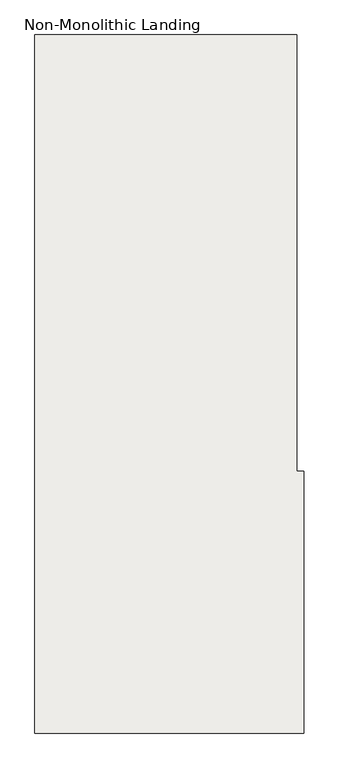
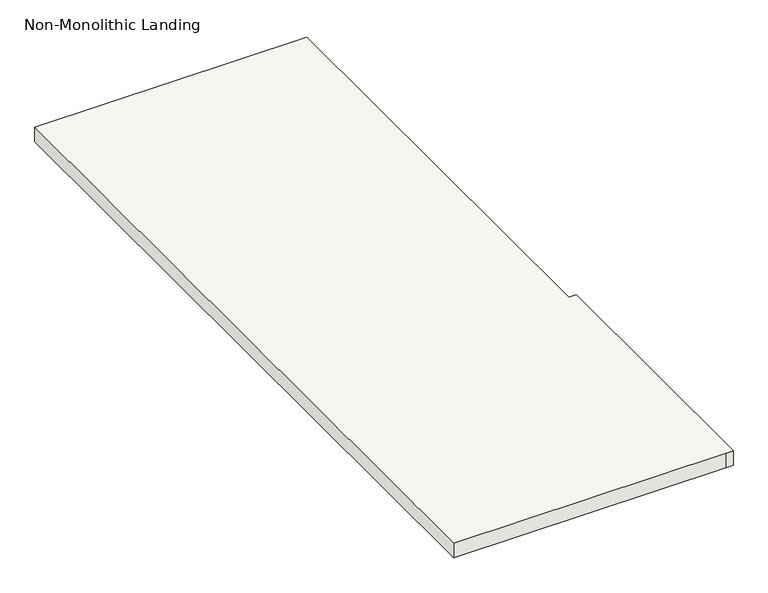
"""IFC4 building model written with IfcOpenShell, lengths in millimetres: slab geometry, Non-Monolithic Landing."""

from ifc_helpers import new_model, si_unit, origin, place, context, project, spatial, faceted_brep, source, transform, mapped, element, save


def non_monolithic_landing_2594b9d5(model_context):
    return source(origin(), model_context, "Body", "Brep", [
        faceted_brep([(-8277.8763529, -1051.6338022, 5010.15), (-8252.4763529, -1051.6338022, 5035.55), (-8252.4763529, -1966.0338022, 5035.55), (-8277.8763529, -1966.0338022, 5010.15), (-9166.8763529, -1051.6338022, 5054.6), (-9166.8763529, -3490.0338022, 5054.6), (-8252.4763529, -3490.0338022, 5054.6), (-8227.0763529, -3490.0338022, 5054.6), (-8227.0763529, -2575.6338022, 5054.6), (-8252.4763529, -2575.6338022, 5054.6), (-8252.4763529, -1051.6338022, 5054.6), (-8277.8763529, -1966.0338022, 5003.8), (-8252.4763529, -1966.0338022, 5003.8), (-8252.4763529, -2575.6338022, 5003.8), (-8227.0763529, -2575.6338022, 5003.8), (-8227.0763529, -3490.0338022, 5003.8), (-8252.4763529, -3490.0338022, 5003.8), (-9166.8763529, -3490.0338022, 5003.8), (-9166.8763529, -1051.6338022, 5003.8), (-8277.8763529, -1051.6338022, 5003.8)], [[[0, 1, 2, 3]], [[4, 5, 6, 7, 8, 9, 10]], [[11, 12, 13, 14, 15, 16, 17, 18, 19]], [[12, 11, 3, 2]], [[11, 19, 0, 3]], [[4, 10, 1, 0, 19, 18]], [[5, 4, 18, 17]], [[6, 5, 17, 16]], [[7, 6, 16, 15]], [[8, 7, 15, 14]], [[9, 8, 14, 13]], [[10, 9, 13, 12, 2, 1]]]),
    ])


if __name__ == "__main__":
    model = new_model("IFC4")
    model_context = context("Model", 3, world=origin())
    ifc_project = project(units=[si_unit("LENGTHUNIT", "METRE", prefix="MILLI")], contexts=[model_context])
    site = spatial("IfcSite", under=ifc_project)
    building = spatial("IfcBuilding", under=site)
    placement = place(None, origin())
    non_monolithic_landing_shape = non_monolithic_landing_2594b9d5(model_context)
    element("IfcSlab", 1, ObjectType="Non-Monolithic Landing", at=placement, inside=building, context=model_context, shape_type="MappedRepresentation", body=[
        mapped(non_monolithic_landing_shape, transform((0.0, 0.0, 0.0), x_axis=(1.0, 0.0, 0.0), y_axis=(0.0, 1.0, 0.0), z_axis=(0.0, 0.0, 1.0))),
    ])
    save(model, "model.ifc")
